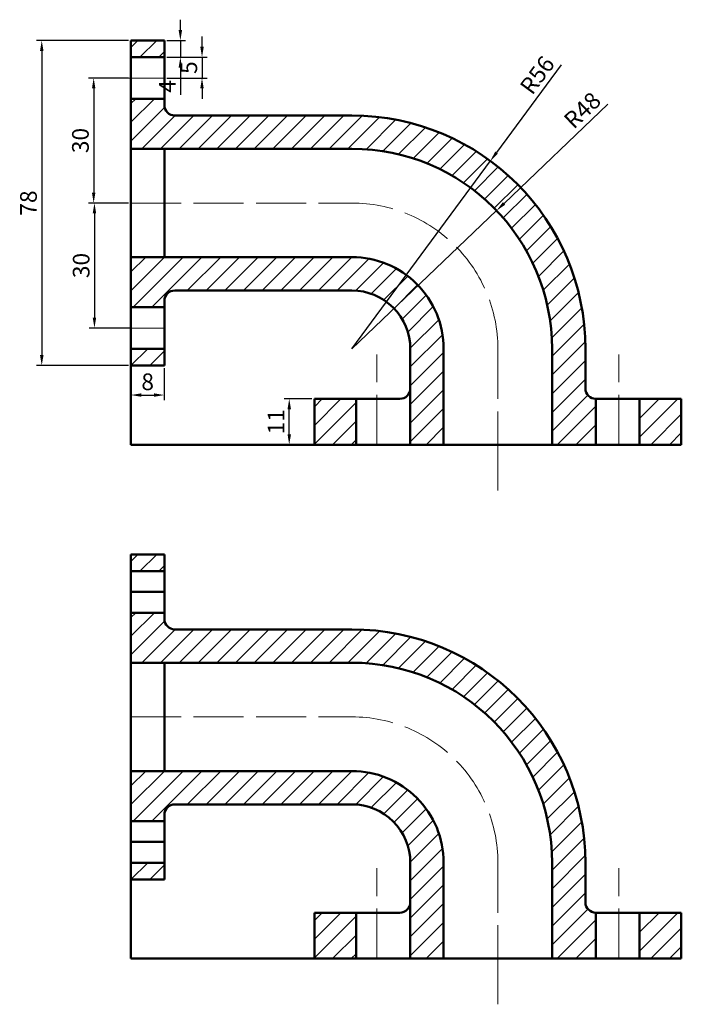
# Model space of a CAD drawing. Units: millimetres. Extents: x 2477 to 2636, y 2000 to 2236.
import ezdxf

# ---------------------------------------------------------------- set-up
doc = ezdxf.new("R2010")
doc.units = ezdxf.units.MM
doc.linetypes.add('ACAD_ISO02W100', pattern=[15, 12, -3])
for name, color, linetype, lineweight in [('M-CNTR', 1, 'ACAD_ISO02W100', 18), ('M-DIMS', 2, 'Continuous', 25), ('M-HATC', 8, 'Continuous', 18), ('M-OUTL', 7, 'Continuous', 50)]:
    doc.layers.add(name, color=color, linetype=linetype, lineweight=lineweight)
doc.styles.get("Standard").update_dxf_attribs({"font": 'arial.ttf'})
doc.dimstyles.new('ISO-25', dxfattribs={"dimtxt": 4, "dimasz": 2.5, "dimexe": 1.25, "dimexo": 0.625, "dimtad": 1, "dimdsep": 46, "dimtxsty": 'Standard', "dimcen": 2.5, "dimadec": 0, "dimazin": 0, "dimtfac": 1, "dimtmove": 0, "dimatfit": 3, "dimfxl": 1, "dimarcsym": 0})

# ---------------------------------------------------------------- blocks, each defined once
blk = doc.blocks.new('*D1')
at = {"layer": 'Defpoints', "color": 0, "transparency": 16777216}
for p in [(2511.65, 2231.42), (2511.65, 2227.42), (2515.5, 2227.42)]:
    blk.add_point(p, dxfattribs=at)
at = {"layer": 'M-DIMS', "color": 0, "lineweight": -2, "transparency": 16777216}
for p, q in [((2515.5, 2233.92), (2515.5, 2236.42)), ((2512.28, 2231.42), (2516.75, 2231.42)), ((2515.5, 2231.42), (2515.5, 2227.42)), ((2512.28, 2227.42), (2516.75, 2227.42)), ((2515.5, 2224.92), (2515.5, 2218.41))]:
    blk.add_line(p, q, dxfattribs=at)
at = {"layer": 'M-DIMS', "color": 0, "transparency": 16777216}
for points in [[(2515.08, 2233.92), (2515.91, 2233.92), (2515.5, 2231.42)], [(2515.08, 2224.92), (2515.91, 2224.92), (2515.5, 2227.42)]]:
    blk.add_solid(points, dxfattribs=at)
at = {"layer": 'M-DIMS', "color": 0, "transparency": 16777216, "insert": (2512.87, 2220.42), "char_height": 4, "attachment_point": 5, "rotation": 90}
blk.add_mtext('4', dxfattribs=at)
blk = doc.blocks.new('*D2')
at = {"layer": 'Defpoints', "color": 0, "transparency": 16777216}
for p in [(2511.65, 2227.42), (2511.65, 2222.42), (2520.69, 2222.42)]:
    blk.add_point(p, dxfattribs=at)
at = {"layer": 'M-DIMS', "color": 0, "lineweight": -2, "transparency": 16777216}
for p, q in [((2520.69, 2229.92), (2520.69, 2232.42)), ((2512.28, 2227.42), (2521.94, 2227.42)), ((2520.69, 2227.42), (2520.69, 2222.42)), ((2512.28, 2222.42), (2521.94, 2222.42)), ((2520.69, 2219.92), (2520.69, 2217.42))]:
    blk.add_line(p, q, dxfattribs=at)
at = {"layer": 'M-DIMS', "color": 0, "transparency": 16777216}
for points in [[(2520.27, 2229.92), (2521.1, 2229.92), (2520.69, 2227.42)], [(2520.27, 2219.92), (2521.1, 2219.92), (2520.69, 2222.42)]]:
    blk.add_solid(points, dxfattribs=at)
at = {"layer": 'M-DIMS', "color": 0, "transparency": 16777216, "insert": (2518.03, 2224.92), "char_height": 4, "attachment_point": 5, "rotation": 90}
blk.add_mtext('5', dxfattribs=at)
blk = doc.blocks.new('*D3')
at = {"layer": 'Defpoints', "color": 0, "transparency": 16777216}
for p in [(2503.65, 2231.42), (2482.25, 2153.42), (2503.65, 2153.42)]:
    blk.add_point(p, dxfattribs=at)
at = {"layer": 'M-DIMS', "color": 0, "lineweight": -2, "transparency": 16777216}
for p, q in [((2503.03, 2231.42), (2481, 2231.42)), ((2482.25, 2228.92), (2482.25, 2155.92)), ((2503.03, 2153.42), (2481, 2153.42))]:
    blk.add_line(p, q, dxfattribs=at)
at = {"layer": 'M-DIMS', "color": 0, "transparency": 16777216}
for points in [[(2481.83, 2228.92), (2482.67, 2228.92), (2482.25, 2231.42)], [(2481.83, 2155.92), (2482.67, 2155.92), (2482.25, 2153.42)]]:
    blk.add_solid(points, dxfattribs=at)
at = {"layer": 'M-DIMS', "color": 0, "transparency": 16777216, "insert": (2479.58, 2192.42), "char_height": 4, "attachment_point": 5, "rotation": 90}
blk.add_mtext('78', dxfattribs=at)
blk = doc.blocks.new('*D4')
at = {"layer": 'Defpoints', "color": 0, "transparency": 16777216}
for p in [(2591.34, 2190.6), (2556.65, 2157.42)]:
    blk.add_point(p, dxfattribs=at)
at = {"layer": 'M-DIMS', "color": 0, "lineweight": -2, "transparency": 16777216}
for p, q in [((2618.02, 2216.13), (2593.14, 2192.33)), ((2556.65, 2157.42), (2591.34, 2190.6))]:
    blk.add_line(p, q, dxfattribs=at)
at = {"layer": 'M-DIMS', "color": 0, "transparency": 16777216}
blk.add_solid([(2592.85, 2192.63), (2593.43, 2192.03), (2591.34, 2190.6)], dxfattribs=at)
at = {"layer": 'M-DIMS', "color": 0, "transparency": 16777216, "insert": (2612.27, 2214.32), "char_height": 4, "attachment_point": 5, "rotation": 43.7304}
blk.add_mtext('R48', dxfattribs=at)
blk = doc.blocks.new('*D5')
at = {"layer": 'Defpoints', "color": 0, "transparency": 16777216}
for p in [(2589.86, 2202.52), (2556.65, 2157.42)]:
    blk.add_point(p, dxfattribs=at)
at = {"layer": 'M-DIMS', "color": 0, "lineweight": -2, "transparency": 16777216}
for p, q in [((2606.86, 2225.6), (2591.34, 2204.53)), ((2556.65, 2157.42), (2589.86, 2202.52))]:
    blk.add_line(p, q, dxfattribs=at)
at = {"layer": 'M-DIMS', "color": 0, "transparency": 16777216}
blk.add_solid([(2591.01, 2204.78), (2591.68, 2204.28), (2589.86, 2202.52)], dxfattribs=at)
at = {"layer": 'M-DIMS', "color": 0, "transparency": 16777216, "insert": (2601.51, 2222.83), "char_height": 4, "attachment_point": 5, "rotation": 53.6303}
blk.add_mtext('R56', dxfattribs=at)
blk = doc.blocks.new('*D6')
at = {"layer": 'Defpoints', "color": 0, "transparency": 16777216}
for p in [(2503.65, 2153.42), (2511.65, 2153.42), (2511.65, 2146.34)]:
    blk.add_point(p, dxfattribs=at)
at = {"layer": 'M-DIMS', "color": 0, "lineweight": -2, "transparency": 16777216}
for p, q in [((2503.65, 2152.8), (2503.65, 2145.09)), ((2511.65, 2152.8), (2511.65, 2145.09)), ((2506.15, 2146.34), (2509.15, 2146.34))]:
    blk.add_line(p, q, dxfattribs=at)
at = {"layer": 'M-DIMS', "color": 0, "transparency": 16777216}
for points in [[(2506.15, 2146.75), (2506.15, 2145.92), (2503.65, 2146.34)], [(2509.15, 2146.75), (2509.15, 2145.92), (2511.65, 2146.34)]]:
    blk.add_solid(points, dxfattribs=at)
at = {"layer": 'M-DIMS', "color": 0, "transparency": 16777216, "insert": (2507.65, 2149), "char_height": 4, "attachment_point": 5}
blk.add_mtext('8', dxfattribs=at)
blk = doc.blocks.new('*D7')
at = {"layer": 'Defpoints', "color": 0, "transparency": 16777216}
for p in [(2541.61, 2145.42), (2547.65, 2145.42), (2547.65, 2134.42)]:
    blk.add_point(p, dxfattribs=at)
at = {"layer": 'M-DIMS', "color": 0, "lineweight": -2, "transparency": 16777216}
for p, q in [((2547.03, 2145.42), (2540.36, 2145.42)), ((2541.61, 2136.92), (2541.61, 2142.92)), ((2547.03, 2134.42), (2540.36, 2134.42))]:
    blk.add_line(p, q, dxfattribs=at)
at = {"layer": 'M-DIMS', "color": 0, "transparency": 16777216}
for points in [[(2541.2, 2142.92), (2542.03, 2142.92), (2541.61, 2145.42)], [(2541.2, 2136.92), (2542.03, 2136.92), (2541.61, 2134.42)]]:
    blk.add_solid(points, dxfattribs=at)
at = {"layer": 'M-DIMS', "color": 0, "transparency": 16777216, "insert": (2538.98, 2139.92), "char_height": 4, "attachment_point": 5, "rotation": 90}
blk.add_mtext('11', dxfattribs=at)
blk = doc.blocks.new('*D8')
at = {"layer": 'Defpoints', "color": 0, "transparency": 16777216}
for p in [(2503.65, 2222.42), (2494.7, 2192.42), (2503.65, 2192.42)]:
    blk.add_point(p, dxfattribs=at)
at = {"layer": 'M-DIMS', "color": 0, "lineweight": -2, "transparency": 16777216}
for p, q in [((2503.03, 2222.42), (2493.45, 2222.42)), ((2494.7, 2219.92), (2494.7, 2194.92)), ((2503.03, 2192.42), (2493.45, 2192.42))]:
    blk.add_line(p, q, dxfattribs=at)
at = {"layer": 'M-DIMS', "color": 0, "transparency": 16777216}
for points in [[(2494.29, 2219.92), (2495.12, 2219.92), (2494.7, 2222.42)], [(2494.29, 2194.92), (2495.12, 2194.92), (2494.7, 2192.42)]]:
    blk.add_solid(points, dxfattribs=at)
at = {"layer": 'M-DIMS', "color": 0, "transparency": 16777216, "insert": (2492.04, 2207.42), "char_height": 4, "attachment_point": 5, "rotation": 90}
blk.add_mtext('30', dxfattribs=at)
blk = doc.blocks.new('*D9')
at = {"layer": 'Defpoints', "color": 0, "transparency": 16777216}
for p in [(2503.65, 2192.42), (2494.89, 2162.42), (2504.12, 2162.42)]:
    blk.add_point(p, dxfattribs=at)
at = {"layer": 'M-DIMS', "color": 0, "lineweight": -2, "transparency": 16777216}
for p, q in [((2503.03, 2192.42), (2493.64, 2192.42)), ((2494.89, 2189.92), (2494.89, 2164.92)), ((2503.49, 2162.42), (2493.64, 2162.42))]:
    blk.add_line(p, q, dxfattribs=at)
at = {"layer": 'M-DIMS', "color": 0, "transparency": 16777216}
for points in [[(2494.47, 2189.92), (2495.3, 2189.92), (2494.89, 2192.42)], [(2494.47, 2164.92), (2495.3, 2164.92), (2494.89, 2162.42)]]:
    blk.add_solid(points, dxfattribs=at)
at = {"layer": 'M-DIMS', "color": 0, "transparency": 16777216, "insert": (2492.22, 2177.42), "char_height": 4, "attachment_point": 5, "rotation": 90}
blk.add_mtext('30', dxfattribs=at)

msp = doc.modelspace()

# ---------------------------------------------------------------- hatches: boundary and pattern name
at = {"layer": 'M-HATC'}
h = msp.add_hatch(dxfattribs=at)
h.set_pattern_fill('ANSI31', color=256)
h.paths.add_polyline_path([(2556.651, 2213.424), (2514.151, 2213.424, -0.4142136), (2511.651, 2215.924), (2511.651, 2217.424), (2503.651, 2217.424), (2503.651, 2205.424), (2556.651, 2205.424, -0.4142136), (2604.651, 2157.424), (2604.651, 2134.424), (2613.651, 2134.424), (2615.151, 2134.424), (2615.151, 2145.424, -0.4142136), (2612.651, 2147.924), (2612.651, 2157.424, 0.4142136)])
h.paths.add_polyline_path([(2556.651, 2179.424), (2503.651, 2179.424), (2503.651, 2167.424), (2511.651, 2167.424), (2511.651, 2168.924, -0.4142136), (2514.151, 2171.424), (2556.651, 2171.424, -0.4142136), (2570.651, 2157.424), (2570.651, 2134.424), (2578.651, 2134.424), (2578.651, 2157.424, 0.4142136)], flags=17)
h.paths.add_polyline_path([(2511.651, 2157.424), (2503.651, 2157.424), (2503.651, 2153.424), (2511.651, 2153.424)], flags=16)
h.paths.add_polyline_path([(2511.651, 2231.424), (2503.651, 2231.424), (2503.651, 2227.419), (2511.651, 2227.419), (2511.651, 2227.424)])
h.paths.add_polyline_path([(2557.651, 2145.424), (2547.651, 2145.424), (2547.651, 2134.424), (2557.651, 2134.424)], flags=16)
h.paths.add_polyline_path([(2635.651, 2145.424), (2625.651, 2145.424), (2625.651, 2134.424), (2635.651, 2134.424)])
h = msp.add_hatch(dxfattribs=at)
h.set_pattern_fill('ANSI31', color=256)
h.set_pattern_definition([(45, (0, -123.3305), (-2.245064, 2.245064), [])])
h.paths.add_polyline_path([(2556.651, 2090.093), (2514.151, 2090.093, -0.4142136), (2511.651, 2092.593), (2511.651, 2094.093), (2503.651, 2094.093), (2503.651, 2082.093), (2556.651, 2082.093, -0.4142136), (2604.651, 2034.093), (2604.651, 2011.093), (2613.651, 2011.093), (2615.151, 2011.093), (2615.151, 2022.093, -0.4142136), (2612.651, 2024.593), (2612.651, 2034.093, 0.4142136)])
h.paths.add_polyline_path([(2556.651, 2056.093), (2503.651, 2056.093), (2503.651, 2044.093), (2511.651, 2044.093), (2511.651, 2045.593, -0.4142136), (2514.151, 2048.093), (2556.651, 2048.093, -0.4142136), (2570.651, 2034.093), (2570.651, 2011.093), (2578.651, 2011.093), (2578.651, 2034.093, 0.4142136)], flags=17)
h.paths.add_polyline_path([(2511.651, 2034.093), (2503.651, 2034.093), (2503.651, 2030.093), (2511.651, 2030.093)], flags=16)
h.paths.add_polyline_path([(2511.651, 2108.093), (2503.651, 2108.093), (2503.651, 2104.089), (2511.651, 2104.089), (2511.651, 2104.093)])
h.paths.add_polyline_path([(2557.651, 2022.093), (2547.651, 2022.093), (2547.651, 2011.093), (2557.651, 2011.093)], flags=16)
h.paths.add_polyline_path([(2635.651, 2022.093), (2625.651, 2022.093), (2625.651, 2011.093), (2635.651, 2011.093)])

# ---------------------------------------------------------------- linework, layer by layer
at = {"layer": 'M-CNTR'}
for p, q in [((2511.651, 2222.424), (2496.587, 2222.424)), ((2511.651, 2162.424), (2496.587, 2162.424)), ((2562.651, 2134.424), (2562.651, 2156.076)), ((2620.651, 2134.424), (2620.651, 2156.076)), ((2591.651, 2134.424), (2591.651, 2123.436)), ((2591.651, 2134.424), (2591.651, 2123.436)), ((2562.651, 2011.093), (2562.651, 2032.746)), ((2620.651, 2011.093), (2620.651, 2032.746)), ((2591.651, 2011.093), (2591.651, 2000.105)), ((2591.651, 2011.093), (2591.651, 2000.105))]:
    msp.add_line(p, q, dxfattribs=at)
for points in [[(2503.651, 2192.424), (2556.651, 2192.424, -0.4142136), (2591.651, 2157.424), (2591.651, 2134.424)], [(2503.651, 2069.093), (2556.651, 2069.093, -0.4142136), (2591.651, 2034.093), (2591.651, 2011.093)]]:
    msp.add_lwpolyline(points, format="xyb", dxfattribs=at)
at = {"layer": 'M-OUTL'}
for p, q in [((2503.651, 2231.424), (2503.651, 2227.424)), ((2503.651, 2231.424), (2511.651, 2231.424)), ((2503.651, 2231.424), (2503.651, 2153.424)), ((2511.651, 2231.424), (2511.651, 2227.424)), ((2503.651, 2227.424), (2503.651, 2222.424)), ((2511.651, 2227.419), (2503.651, 2227.419)), ((2511.651, 2227.424), (2511.651, 2222.424)), ((2511.651, 2222.424), (2511.651, 2217.424)), ((2511.651, 2217.424), (2503.651, 2217.424)), ((2511.651, 2217.424), (2511.651, 2215.924)), ((2514.151, 2213.424), (2556.651, 2213.424)), ((2503.651, 2205.424), (2556.651, 2205.424)), ((2511.651, 2179.424), (2511.651, 2205.424)), ((2503.651, 2192.424), (2503.651, 2134.424)), ((2511.651, 2167.424), (2503.651, 2167.424)), ((2511.651, 2162.424), (2511.651, 2167.424)), ((2511.651, 2157.424), (2511.651, 2162.424)), ((2511.651, 2157.424), (2503.651, 2157.424)), ((2511.651, 2153.424), (2511.651, 2157.424)), ((2604.651, 2134.424), (2604.651, 2157.424)), ((2612.651, 2147.924), (2612.651, 2157.424)), ((2503.651, 2153.424), (2511.651, 2153.424)), ((2547.651, 2134.424), (2547.651, 2145.424)), ((2547.651, 2145.424), (2562.651, 2145.424)), ((2557.651, 2134.424), (2557.651, 2145.424)), ((2568.151, 2145.424), (2562.651, 2145.424)), ((2615.151, 2145.424), (2620.651, 2145.424)), ((2615.151, 2145.424), (2615.151, 2134.424)), ((2635.651, 2145.424), (2620.651, 2145.424)), ((2625.651, 2134.424), (2625.651, 2145.424)), ((2635.651, 2134.424), (2635.651, 2145.424)), ((2503.651, 2134.424), (2591.651, 2134.424)), ((2578.651, 2134.424), (2569.651, 2134.424)), ((2591.651, 2134.424), (2620.651, 2134.424)), ((2604.651, 2134.424), (2613.651, 2134.424)), ((2620.651, 2134.424), (2635.651, 2134.424)), ((2620.651, 2134.424), (2635.651, 2134.424)), ((2635.651, 2134.424), (2625.651, 2134.424)), ((2503.651, 2108.093), (2503.651, 2104.093)), ((2503.651, 2108.093), (2511.651, 2108.093)), ((2503.651, 2108.093), (2503.651, 2030.093)), ((2511.651, 2108.093), (2511.651, 2104.093)), ((2503.651, 2104.093), (2503.651, 2099.093)), ((2511.651, 2104.089), (2503.651, 2104.089)), ((2511.651, 2104.093), (2511.651, 2099.093)), ((2511.651, 2099.093), (2503.651, 2099.093)), ((2511.651, 2099.093), (2511.651, 2094.093)), ((2511.651, 2094.093), (2503.651, 2094.093)), ((2511.651, 2094.093), (2511.651, 2092.593)), ((2514.151, 2090.093), (2556.651, 2090.093)), ((2503.651, 2082.093), (2556.651, 2082.093)), ((2511.651, 2056.093), (2511.651, 2082.093)), ((2503.651, 2069.093), (2503.651, 2011.093)), ((2511.651, 2044.093), (2503.651, 2044.093)), ((2511.651, 2039.093), (2511.651, 2044.093)), ((2511.651, 2039.093), (2503.651, 2039.093)), ((2511.651, 2034.093), (2511.651, 2039.093)), ((2511.651, 2034.093), (2503.651, 2034.093)), ((2511.651, 2030.093), (2511.651, 2034.093)), ((2604.651, 2011.093), (2604.651, 2034.093)), ((2612.651, 2024.593), (2612.651, 2034.093)), ((2503.651, 2030.093), (2511.651, 2030.093)), ((2547.651, 2011.093), (2547.651, 2022.093)), ((2547.651, 2022.093), (2562.651, 2022.093)), ((2557.651, 2011.093), (2557.651, 2022.093)), ((2568.151, 2022.093), (2562.651, 2022.093)), ((2615.151, 2022.093), (2620.651, 2022.093)), ((2615.151, 2022.093), (2615.151, 2011.093)), ((2635.651, 2022.093), (2620.651, 2022.093)), ((2625.651, 2011.093), (2625.651, 2022.093)), ((2635.651, 2011.093), (2635.651, 2022.093)), ((2503.651, 2011.093), (2591.651, 2011.093)), ((2557.651, 2011.093), (2562.651, 2011.093)), ((2578.651, 2011.093), (2569.651, 2011.093)), ((2591.651, 2011.093), (2620.651, 2011.093)), ((2604.651, 2011.093), (2613.651, 2011.093)), ((2620.651, 2011.093), (2635.651, 2011.093)), ((2620.651, 2011.093), (2635.651, 2011.093)), ((2635.651, 2011.093), (2625.651, 2011.093))]:
    msp.add_line(p, q, dxfattribs=at)
for points in [[(2503.651, 2179.424), (2556.651, 2179.424, -0.4142136), (2578.651, 2157.424), (2578.651, 2134.424)], [(2511.651, 2167.424), (2511.651, 2168.924, -0.4142136), (2514.151, 2171.424), (2556.651, 2171.424, -0.4142136), (2570.651, 2157.424), (2570.651, 2134.424)], [(2503.651, 2056.093), (2556.651, 2056.093, -0.4142136), (2578.651, 2034.093), (2578.651, 2011.093)], [(2511.651, 2044.093), (2511.651, 2045.593, -0.4142136), (2514.151, 2048.093), (2556.651, 2048.093, -0.4142136), (2570.651, 2034.093), (2570.651, 2011.093)]]:
    msp.add_lwpolyline(points, format="xyb", dxfattribs=at)
for centre, radius, start, end in [((2514.151, 2215.924), 2.5, 180, 270), ((2556.651, 2157.424), 56, 0, 90), ((2556.651, 2157.424), 48, 0, 90), ((2568.151, 2147.924), 2.5, 270, 0), ((2615.151, 2147.924), 2.5, 180, 270), ((2514.151, 2092.593), 2.5, 180, 270), ((2556.651, 2034.093), 56, 0, 90), ((2556.651, 2034.093), 48, 0, 90), ((2568.151, 2024.593), 2.5, 270, 0), ((2615.151, 2024.593), 2.5, 180, 270)]:
    msp.add_arc(centre, radius, start, end, dxfattribs=at)

# ---------------------------------------------------------------- dimensions: what is measured, and where the dimension line sits
at = {"layer": 'M-DIMS'}
for base, p1, p2, picture, middle in [((2515.498, 2227.424), (2511.651, 2231.424), (2511.651, 2227.424), '*D1', (2512.873, 2220.416)), ((2482.251, 2153.424), (2503.651, 2231.424), (2503.651, 2153.424), '*D3', (2479.584, 2192.424)), ((2520.6863, 2222.4239), (2511.6505, 2227.4191), (2511.6505, 2222.4239), '*D2', (2518.0272, 2224.9215)), ((2494.705, 2192.424), (2503.651, 2222.424), (2503.651, 2192.424), '*D8', (2492.036, 2207.424)), ((2494.886, 2162.424), (2503.651, 2192.424), (2504.119, 2162.424), '*D9', (2492.217, 2177.424)), ((2541.614, 2145.424), (2547.651, 2134.424), (2547.651, 2145.424), '*D7', (2538.981, 2139.924))]:
    dim = msp.add_linear_dim(base=base, p1=p1, p2=p2, angle=90, dimstyle='ISO-25', override={"dimclrd": 0, "dimclre": 0, "dimclrt": 0}, dxfattribs=at)
    dim.commit()
    dim.dimension.update_dxf_attribs({"geometry": picture, "text_midpoint": middle})
for mpoint, picture, middle in [((2589.858, 2202.516), '*D5', (2603.655, 2221.25)), ((2591.335, 2190.605), '*D4', (2614.113, 2212.395))]:
    dim = msp.add_radius_dim(center=(2556.651, 2157.424), mpoint=mpoint, dimstyle='ISO-25', override={"dimclrd": 0, "dimclre": 0, "dimclrt": 0}, dxfattribs=at)
    dim.commit()
    dim.dimension.update_dxf_attribs({"geometry": picture, "text_midpoint": middle, "dimtype": 164})
dim = msp.add_linear_dim(base=(2511.651, 2146.337), p1=(2503.651, 2153.424), p2=(2511.651, 2153.424), dimstyle='ISO-25', override={"dimclrd": 0, "dimclre": 0, "dimclrt": 0}, dxfattribs=at)
dim.commit()
dim.dimension.update_dxf_attribs({"geometry": '*D6', "text_midpoint": (2507.651, 2149.004)})

doc.saveas('drawing.dxf')
